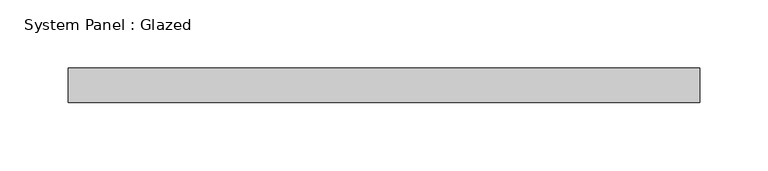
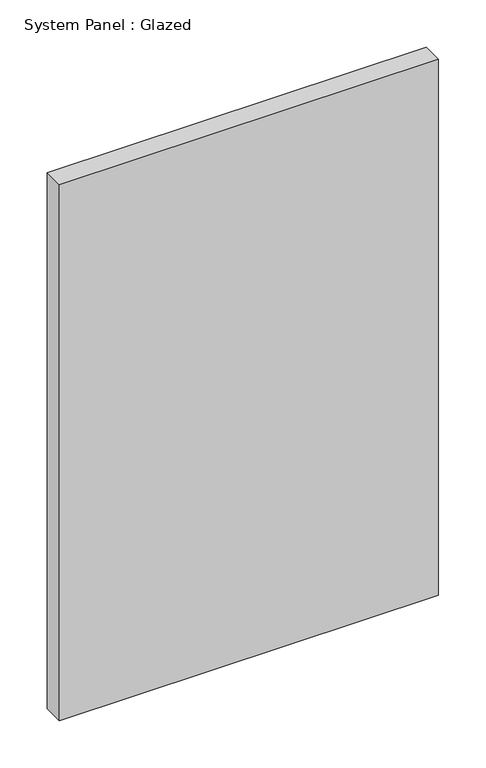
"""IFC4 building model written with IfcOpenShell, lengths in millimetres: plate geometry, System Panel : Glazed."""

from ifc_helpers import new_model, si_unit, origin, origin_with_axes, place, context, project, spatial, polyline, outline, extrude, source, transform, mapped, element, save


def system_panel_glazed_cb1b45af(model_context):
    return source(origin(), model_context, "Body", "SweptSolid", [
        extrude(outline(polyline([(231.775, 19.05), (-231.775, 19.05), (-231.775, 44.45), (231.775, 44.45), (231.775, 19.05)])), origin_with_axes(), (0.0, 0.0, 1.0), 692.9627727),
    ])


if __name__ == "__main__":
    model = new_model("IFC4")
    model_context = context("Model", 3, world=origin())
    ifc_project = project(units=[si_unit("LENGTHUNIT", "METRE", prefix="MILLI")], contexts=[model_context])
    site = spatial("IfcSite", under=ifc_project)
    building = spatial("IfcBuilding", under=site)
    placement = place(None, origin())
    system_panel_glazed_shape = system_panel_glazed_cb1b45af(model_context)
    element("IfcPlate", 1, ObjectType="System Panel : Glazed", at=placement, inside=building, context=model_context, shape_type="MappedRepresentation", body=[
        mapped(system_panel_glazed_shape, transform((0.0, 0.0, 0.0), x_axis=(1.0, 0.0, 0.0), y_axis=(0.0, 1.0, 0.0), z_axis=(0.0, 0.0, 1.0))),
    ])
    save(model, "model.ifc")

# Revit data of these elements
# Type "System Panel : Glazed"
#   Construction Type Id = "GSP4R"
#   Analytic Construction = "1/8 in Pilkington single glazing"
#   Visual Light Transmittance = 0.9
#   Solar Heat Gain Coefficient = 0.86
#   Heat Transfer Coefficient (U) = 1.18115 BTU/(h·ft²·°F)
#   Define Thermal Properties by = 1
# Element 1 (IfcPlate, "System Panel : Glazed")
#   Materials on its faces: "Glass"
# Materials
#   "Glass": class "Glass", colour RGB 0 128 192, transparency 0.75, Description = "Soda Lime Glass", Cost = 0
